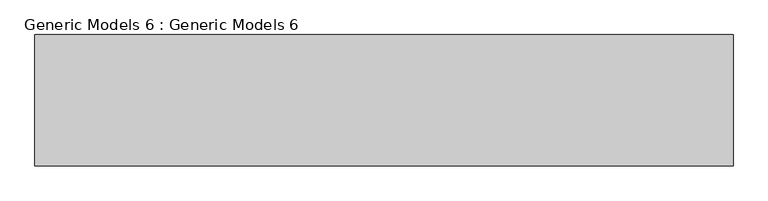
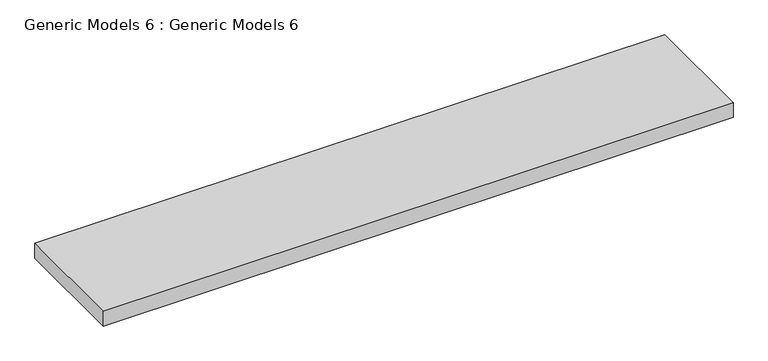
"""IFC4 building model written with IfcOpenShell, lengths in millimetres: proxy geometry, Generic Models 6 : Generic Models 6."""

from ifc_helpers import new_model, si_unit, frame, origin, place, context, project, spatial, polyline, outline, extrude, source, transform, mapped, element, save


def generic_models_6_generic_models_6_873e410b(model_context):
    return source(origin(), model_context, "Body", "SweptSolid", [
        extrude(outline(polyline([(-11735.9777764, -11756.5656885), (11124.0222236, -11756.5656885), (11124.0222236, -16060.0466235), (-11735.9777764, -16060.0466235), (-11735.9777764, -11756.5656885)])), frame((0.0, 0.0, -558.8), z_axis=(0.0, 0.0, 1.0), x_axis=(1.0, 0.0, 0.0)), (0.0, 0.0, 1.0), 558.8),
    ])


if __name__ == "__main__":
    model = new_model("IFC4")
    model_context = context("Model", 3, world=origin())
    ifc_project = project(units=[si_unit("LENGTHUNIT", "METRE", prefix="MILLI")], contexts=[model_context])
    site = spatial("IfcSite", under=ifc_project)
    building = spatial("IfcBuilding", under=site)
    placement = place(None, origin())
    generic_models_6_generic_models_6_shape = generic_models_6_generic_models_6_873e410b(model_context)
    element("IfcBuildingElementProxy", 1, Name="Generic Models 6 : Generic Models 6", ObjectType="Generic Models 6 : Generic Models 6", at=placement, inside=building, context=model_context, shape_type="MappedRepresentation", body=[
        mapped(generic_models_6_generic_models_6_shape, transform((0.0, 0.0, 0.0), x_axis=(1.0, 0.0, 0.0), y_axis=(0.0, 1.0, 0.0), z_axis=(0.0, 0.0, 1.0))),
    ])
    save(model, "model.ifc")
